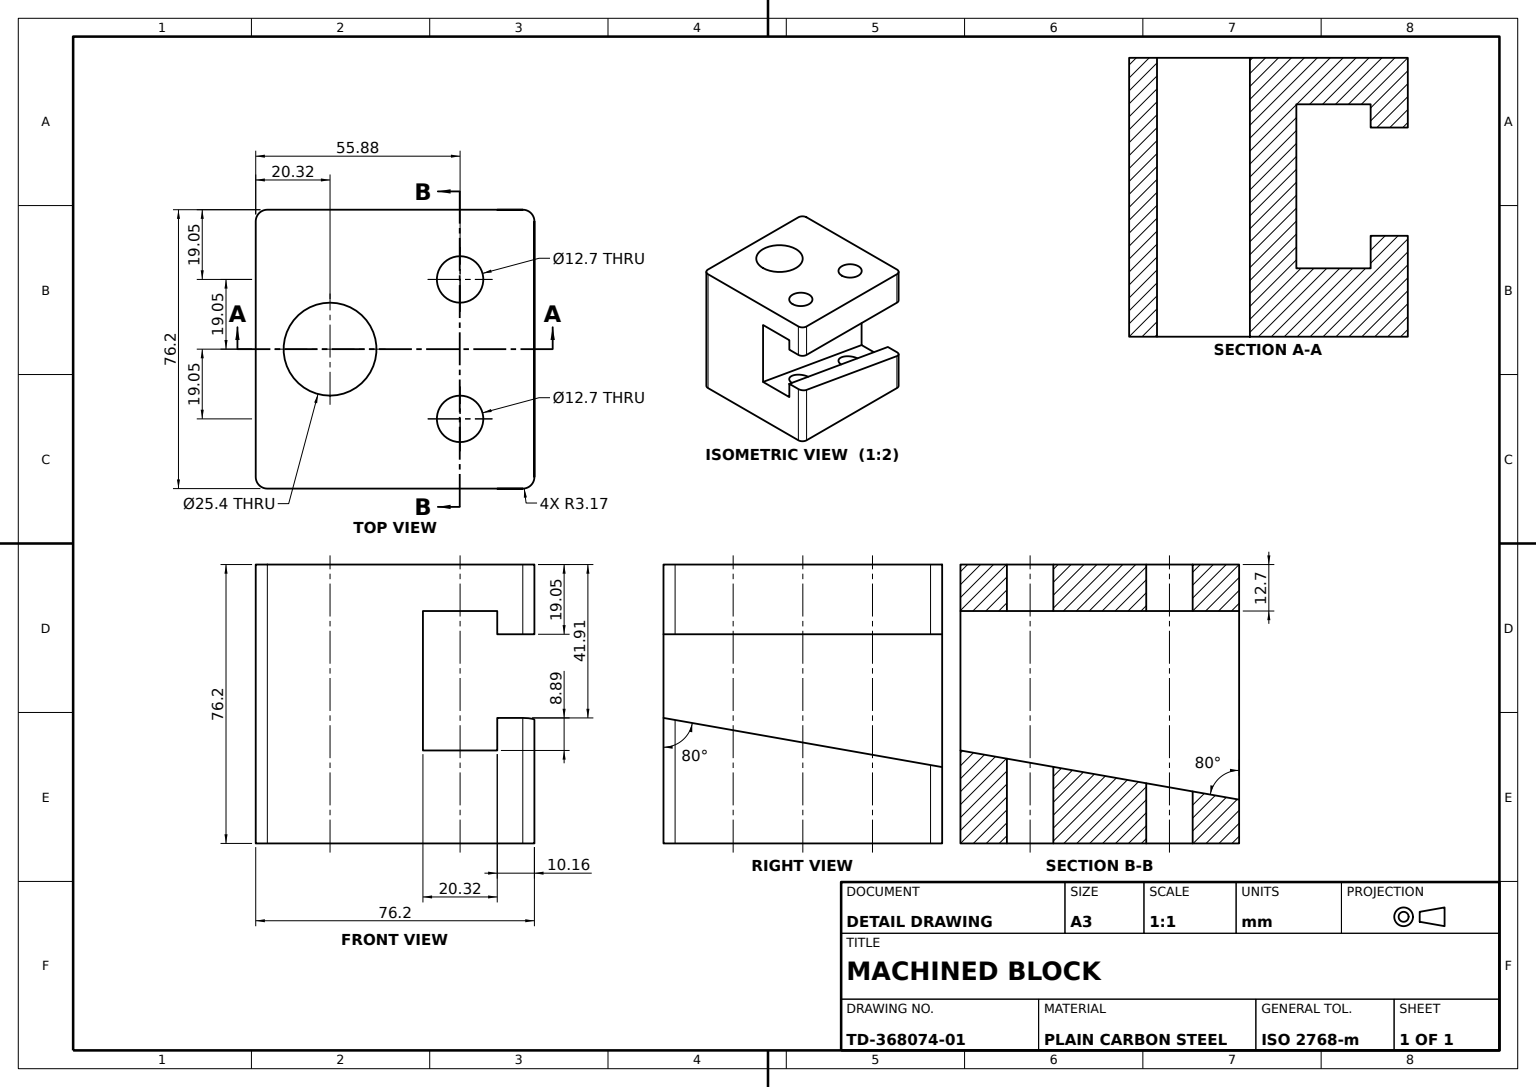
from build123d import *

# Parameters (mm, degrees)
BLOCK_PROFILE_SKETCH_W  = 76.2
BLOCK_PROFILE_SKETCH_H  = 76.2
BLOCK_BODY_3IN_DEPTH    = 38.1
ANGLED_SLOT_CUT_DEPTH   = 10.16
SLOT_UNDERCUT_CUT_DEPTH = 20.32
EDGE_FILLETS_R0_125_R   = 3.175
TOP_HOLES_SKETCH_R      = 6.35
TOP_HOLES_SKETCH_R_2    = 12.7
TOP_HOLES_3X_DEPTH      = 94.3255592


with BuildPart() as part:
    # Block Profile Sketch → Block Body 3in (new, symmetric)
    with BuildSketch(Plane.XY):
        Rectangle(BLOCK_PROFILE_SKETCH_W, BLOCK_PROFILE_SKETCH_H)
    extrude(amount=BLOCK_BODY_3IN_DEPTH, both=True)

    # Angled Slot Sketch → Angled Slot Cut (cut)
    with BuildSketch(Plane.ZY.offset(38.1)):
        Polygon((38.1, -17.24611593), (-38.1, -3.81), (-38.1, 19.05), (38.1, 19.05), align=None)
    extrude(amount=-ANGLED_SLOT_CUT_DEPTH, mode=Mode.SUBTRACT)

    # Slot Undercut Sketch → Slot Undercut Cut (cut)
    with BuildSketch(Plane.ZY.offset(27.94)):
        Polygon((-38.1, 25.4), (38.1, 25.4), (38.1, -26.13611593), (-38.1, -12.7), align=None)
    extrude(amount=-SLOT_UNDERCUT_CUT_DEPTH, mode=Mode.SUBTRACT)

    # Edge Fillets R0.125
    edge_fillets_r0_125_edges = [part.edges().sort_by_distance(p)[0] for p in [
        (-38.1, 28.575, 38.1),
        (-38.1, -20.955, -38.1),
        (-38.1, -27.673057965, 38.1),
        (38.1, 0, 38.1),
        (-38.1, 28.575, -38.1),
        (38.1, 0, -38.1),
    ]]
    fillet(edge_fillets_r0_125_edges, radius=EDGE_FILLETS_R0_125_R)

    # Top Holes Sketch → Top Holes 3x (cut, through all)
    with BuildSketch(Plane(origin=(0, 38.1, 0), x_dir=(1, 0, 0), z_dir=(0, 1, 0))):
        with Locations(Location((-17.78, 19.05, 0), (0, 0, 270))):
            Circle(TOP_HOLES_SKETCH_R)
        with Locations(Location((-17.78, -19.05, 0), (0, 0, 270))):
            Circle(TOP_HOLES_SKETCH_R)
        with Locations(Location((17.78, 0, 0), (0, 0, 270))):
            Circle(TOP_HOLES_SKETCH_R_2)
    extrude(amount=-TOP_HOLES_3X_DEPTH, mode=Mode.SUBTRACT)


solid = part.part
